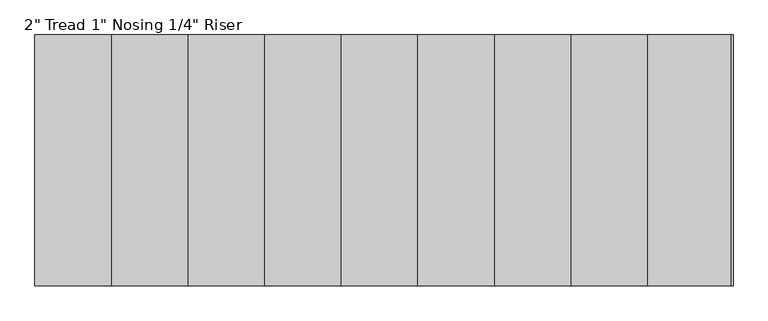
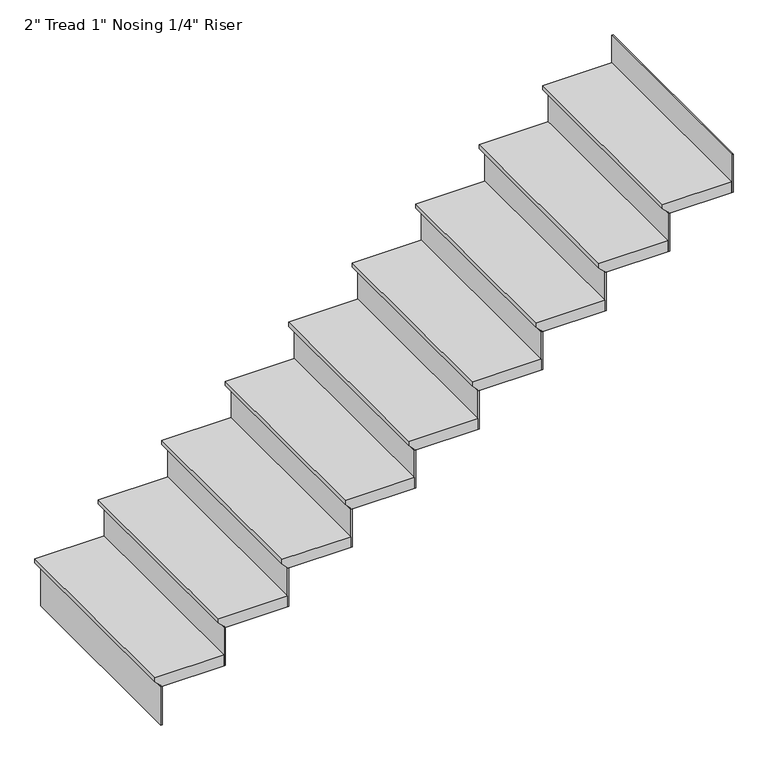
"""IFC4 building model written with IfcOpenShell, lengths in millimetres: stair flight geometry."""

from ifc_helpers import new_model, si_unit, frame, origin, place, context, project, spatial, polyline, outline, extrude, source, transform, mapped, element, save


def stair_flight_fc52eaa6(model_context):
    return source(origin(), model_context, "Body", "SweptSolid", [
        extrude(outline(polyline([(2209.8, 29868.2316163), (2209.8, 29563.4316163), (2190.75, 29563.4316163), (2165.35, 29588.8316163), (2159.0, 29588.8316163), (2159.0, 29868.2316163), (2209.8, 29868.2316163)])), frame((0.0, 7040.8480552, 0.0), z_axis=(0.0, 1.0, 0.0), x_axis=(0.0, 0.0, 1.0)), (0.0, 0.0, 1.0), 914.4),
        extrude(outline(polyline([(29595.1816163, 7040.8480552), (29588.8316163, 7040.8480552), (29588.8316163, 7955.2480552), (29595.1816163, 7955.2480552), (29595.1816163, 7040.8480552)])), frame((0.0, 0.0, 1981.2), z_axis=(0.0, 0.0, 1.0), x_axis=(1.0, 0.0, 0.0)), (0.0, 0.0, 1.0), 177.8),
        extrude(outline(polyline([(29874.5816163, 7040.8480552), (29868.2316163, 7040.8480552), (29868.2316163, 7955.2480552), (29874.5816163, 7955.2480552), (29874.5816163, 7040.8480552)])), frame((0.0, 0.0, 2159.0), z_axis=(0.0, 0.0, 1.0), x_axis=(1.0, 0.0, 0.0)), (0.0, 0.0, 1.0), 177.8),
        extrude(outline(polyline([(2387.6, 30147.6316163), (2387.6, 29842.8316163), (2368.55, 29842.8316163), (2343.15, 29868.2316163), (2336.8, 29868.2316163), (2336.8, 30147.6316163), (2387.6, 30147.6316163)])), frame((0.0, 7040.8480552, 0.0), z_axis=(0.0, 1.0, 0.0), x_axis=(0.0, 0.0, 1.0)), (0.0, 0.0, 1.0), 914.4),
        extrude(outline(polyline([(30153.9816163, 7040.8480552), (30147.6316163, 7040.8480552), (30147.6316163, 7955.2480552), (30153.9816163, 7955.2480552), (30153.9816163, 7040.8480552)])), frame((0.0, 0.0, 2336.8), z_axis=(0.0, 0.0, 1.0), x_axis=(1.0, 0.0, 0.0)), (0.0, 0.0, 1.0), 177.8),
        extrude(outline(polyline([(2565.4, 30427.0316163), (2565.4, 30122.2316163), (2546.35, 30122.2316163), (2520.95, 30147.6316163), (2514.6, 30147.6316163), (2514.6, 30427.0316163), (2565.4, 30427.0316163)])), frame((0.0, 7040.8480552, 0.0), z_axis=(0.0, 1.0, 0.0), x_axis=(0.0, 0.0, 1.0)), (0.0, 0.0, 1.0), 914.4),
        extrude(outline(polyline([(30433.3816163, 7040.8480552), (30427.0316163, 7040.8480552), (30427.0316163, 7955.2480552), (30433.3816163, 7955.2480552), (30433.3816163, 7040.8480552)])), frame((0.0, 0.0, 2514.6), z_axis=(0.0, 0.0, 1.0), x_axis=(1.0, 0.0, 0.0)), (0.0, 0.0, 1.0), 177.8),
        extrude(outline(polyline([(2743.2, 30706.4316163), (2743.2, 30401.6316163), (2724.15, 30401.6316163), (2698.75, 30427.0316163), (2692.4, 30427.0316163), (2692.4, 30706.4316163), (2743.2, 30706.4316163)])), frame((0.0, 7040.8480552, 0.0), z_axis=(0.0, 1.0, 0.0), x_axis=(0.0, 0.0, 1.0)), (0.0, 0.0, 1.0), 914.4),
        extrude(outline(polyline([(30712.7816163, 7040.8480552), (30706.4316163, 7040.8480552), (30706.4316163, 7955.2480552), (30712.7816163, 7955.2480552), (30712.7816163, 7040.8480552)])), frame((0.0, 0.0, 2692.4), z_axis=(0.0, 0.0, 1.0), x_axis=(1.0, 0.0, 0.0)), (0.0, 0.0, 1.0), 177.8),
        extrude(outline(polyline([(2921.0, 30985.8316163), (2921.0, 30681.0316163), (2901.95, 30681.0316163), (2876.55, 30706.4316163), (2870.2, 30706.4316163), (2870.2, 30985.8316163), (2921.0, 30985.8316163)])), frame((0.0, 7040.8480552, 0.0), z_axis=(0.0, 1.0, 0.0), x_axis=(0.0, 0.0, 1.0)), (0.0, 0.0, 1.0), 914.4),
        extrude(outline(polyline([(30992.1816163, 7040.8480552), (30985.8316163, 7040.8480552), (30985.8316163, 7955.2480552), (30992.1816163, 7955.2480552), (30992.1816163, 7040.8480552)])), frame((0.0, 0.0, 2870.2), z_axis=(0.0, 0.0, 1.0), x_axis=(1.0, 0.0, 0.0)), (0.0, 0.0, 1.0), 177.8),
        extrude(outline(polyline([(3098.8, 31265.2316163), (3098.8, 30960.4316163), (3079.75, 30960.4316163), (3054.35, 30985.8316163), (3048.0, 30985.8316163), (3048.0, 31265.2316163), (3098.8, 31265.2316163)])), frame((0.0, 7040.8480552, 0.0), z_axis=(0.0, 1.0, 0.0), x_axis=(0.0, 0.0, 1.0)), (0.0, 0.0, 1.0), 914.4),
        extrude(outline(polyline([(31271.5816163, 7040.8480552), (31265.2316163, 7040.8480552), (31265.2316163, 7955.2480552), (31271.5816163, 7955.2480552), (31271.5816163, 7040.8480552)])), frame((0.0, 0.0, 3048.0), z_axis=(0.0, 0.0, 1.0), x_axis=(1.0, 0.0, 0.0)), (0.0, 0.0, 1.0), 177.8),
        extrude(outline(polyline([(3276.6, 31544.6316163), (3276.6, 31239.8316163), (3257.55, 31239.8316163), (3232.15, 31265.2316163), (3225.8, 31265.2316163), (3225.8, 31544.6316163), (3276.6, 31544.6316163)])), frame((0.0, 7040.8480552, 0.0), z_axis=(0.0, 1.0, 0.0), x_axis=(0.0, 0.0, 1.0)), (0.0, 0.0, 1.0), 914.4),
        extrude(outline(polyline([(31550.9816163, 7040.8480552), (31544.6316163, 7040.8480552), (31544.6316163, 7955.2480552), (31550.9816163, 7955.2480552), (31550.9816163, 7040.8480552)])), frame((0.0, 0.0, 3225.8), z_axis=(0.0, 0.0, 1.0), x_axis=(1.0, 0.0, 0.0)), (0.0, 0.0, 1.0), 177.8),
        extrude(outline(polyline([(3454.4, 31824.0316163), (3454.4, 31519.2316163), (3435.35, 31519.2316163), (3409.95, 31544.6316163), (3403.6, 31544.6316163), (3403.6, 31824.0316163), (3454.4, 31824.0316163)])), frame((0.0, 7040.8480552, 0.0), z_axis=(0.0, 1.0, 0.0), x_axis=(0.0, 0.0, 1.0)), (0.0, 0.0, 1.0), 914.4),
        extrude(outline(polyline([(31830.3816163, 7040.8480552), (31824.0316163, 7040.8480552), (31824.0316163, 7955.2480552), (31830.3816163, 7955.2480552), (31830.3816163, 7040.8480552)])), frame((0.0, 0.0, 3403.6), z_axis=(0.0, 0.0, 1.0), x_axis=(1.0, 0.0, 0.0)), (0.0, 0.0, 1.0), 177.8),
        extrude(outline(polyline([(32109.7816163, 7040.8480552), (32103.4316163, 7040.8480552), (32103.4316163, 7955.2480552), (32109.7816163, 7955.2480552), (32109.7816163, 7040.8480552)])), frame((0.0, 0.0, 3581.4), z_axis=(0.0, 0.0, 1.0), x_axis=(1.0, 0.0, 0.0)), (0.0, 0.0, 1.0), 177.8),
        extrude(outline(polyline([(3632.2, 32103.4316163), (3632.2, 31798.6316163), (3613.15, 31798.6316163), (3587.75, 31824.0316163), (3581.4, 31824.0316163), (3581.4, 32103.4316163), (3632.2, 32103.4316163)])), frame((0.0, 7040.8480552, 0.0), z_axis=(0.0, 1.0, 0.0), x_axis=(0.0, 0.0, 1.0)), (0.0, 0.0, 1.0), 914.4),
    ])


if __name__ == "__main__":
    model = new_model("IFC4")
    model_context = context("Model", 3, world=origin())
    ifc_project = project(units=[si_unit("LENGTHUNIT", "METRE", prefix="MILLI")], contexts=[model_context])
    site = spatial("IfcSite", under=ifc_project)
    building = spatial("IfcBuilding", under=site)
    placement = place(None, origin())
    stair_flight_shape = stair_flight_fc52eaa6(model_context)
    element("IfcStairFlight", 1, ObjectType="2\" Tread 1\" Nosing 1/4\" Riser", at=placement, inside=building, context=model_context, shape_type="MappedRepresentation", body=[
        mapped(stair_flight_shape, transform((0.0, 0.0, 0.0), x_axis=(1.0, 0.0, 0.0), y_axis=(0.0, 1.0, 0.0), z_axis=(0.0, 0.0, 1.0))),
    ])
    save(model, "model.ifc")
